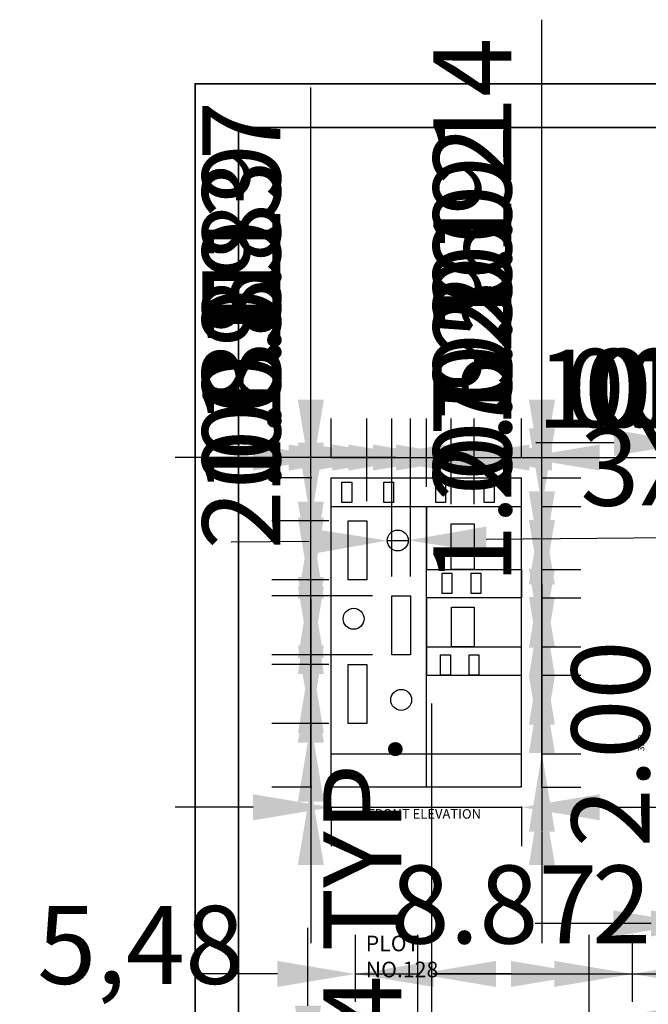
# Model space of a CAD drawing. Units: metres. Extents: x 782 to 1487, y 1262 to 7446.
# Tile 19 of 25: x 782 to 802, y 1313 to 1345. Entities that reach past the tile are written whole.
import ezdxf

# ---------------------------------------------------------------- set-up
doc = ezdxf.new("R2010")
doc.units = ezdxf.units.M
for name, color, linetype, lineweight in [('A-ANNO-DIMS', 2, 'Continuous', 18), ('A-ANNO-TEXT', 3, 'Continuous', 18), ('A-ANNO-TTLB', 7, 'Continuous', 35), ('A-ELEV', 7, 'Continuous', 25)]:
    doc.layers.add(name, color=color, linetype=linetype, lineweight=lineweight)
doc.styles.get("Standard").update_dxf_attribs({"font": 'arial.ttf'})
doc.dimstyles.new('ISO-25', dxfattribs={"dimtxt": 2.5, "dimasz": 2.5, "dimexe": 1.25, "dimexo": 0.625, "dimtad": 1, "dimtxsty": 'Standard', "dimcen": 2.5, "dimadec": 0, "dimazin": 0, "dimtfac": 1, "dimtmove": 0, "dimatfit": 3, "dimfxl": 1, "dimarcsym": 0})

# ---------------------------------------------------------------- blocks, each defined once
blk = doc.blocks.new('*D2')
at = {"layer": 'A-ANNO-DIMS', "color": 0, "lineweight": -2, "transparency": 16777216}
for p, q in [((794.559, 1311.575), (794.559, 1314.2)), ((800.039, 1311.575), (800.039, 1314.2)), ((792.059, 1312.95), (781.81, 1312.95)), ((800.039, 1312.95), (794.559, 1312.95)), ((802.539, 1312.95), (805.039, 1312.95))]:
    blk.add_line(p, q, dxfattribs=at)
at = {"layer": 'A-ANNO-DIMS', "color": 0, "transparency": 16777216}
for points in [[(792.059, 1313.367), (792.059, 1312.534), (794.559, 1312.95)], [(802.539, 1313.367), (802.539, 1312.534), (800.039, 1312.95)]]:
    blk.add_solid(points, dxfattribs=at)
at = {"layer": 'Defpoints', "color": 0, "transparency": 16777216}
for p in [(794.559, 1312.95), (794.559, 1310.95), (800.039, 1310.95)]:
    blk.add_point(p, dxfattribs=at)
at = {"layer": 'A-ANNO-DIMS', "color": 0, "transparency": 16777216, "insert": (785.685, 1315.078), "char_height": 2.5, "width": 6.51678, "attachment_point": 5}
blk.add_mtext('5,48', dxfattribs=at)
blk = doc.blocks.new('*D31')
at = {"layer": 'A-ANNO-DIMS', "color": 0, "lineweight": -2, "transparency": 16777216}
for p, q in [((795.004, 1304.305), (795.004, 1323.137)), ((795.004, 1301.469), (795.004, 1301.805)), ((795.571, 1301.805), (796.254, 1301.805)), ((795.571, 1301.469), (796.254, 1301.469)), ((795.004, 1298.969), (795.004, 1296.469))]:
    blk.add_line(p, q, dxfattribs=at)
at = {"layer": 'A-ANNO-DIMS', "color": 0, "transparency": 16777216}
for points in [[(794.587, 1304.305), (795.421, 1304.305), (795.004, 1301.805)], [(794.587, 1298.969), (795.421, 1298.969), (795.004, 1301.469)]]:
    blk.add_solid(points, dxfattribs=at)
at = {"layer": 'Defpoints', "color": 0, "transparency": 16777216}
for p in [(794.946, 1301.805), (795.004, 1301.805), (794.946, 1301.469)]:
    blk.add_point(p, dxfattribs=at)
at = {"layer": 'A-ANNO-DIMS', "color": 0, "transparency": 16777216, "insert": (793.102, 1314.971), "char_height": 2.5, "attachment_point": 5, "rotation": 90}
blk.add_mtext('0.34 TYP.', dxfattribs=at)
blk = doc.blocks.new('*D32')
at = {"layer": 'A-ANNO-DIMS', "color": 0, "lineweight": -2, "transparency": 16777216}
for p, q in [((791.039, 1313.45), (791.039, 1315.95)), ((793.934, 1310.95), (789.789, 1310.95)), ((791.039, 1310.95), (791.039, 1306.772)), ((793.934, 1306.772), (789.789, 1306.772)), ((791.039, 1304.272), (791.039, 1291.98))]:
    blk.add_line(p, q, dxfattribs=at)
at = {"layer": 'A-ANNO-DIMS', "color": 0, "transparency": 16777216}
for points in [[(790.622, 1313.45), (791.456, 1313.45), (791.039, 1310.95)], [(790.622, 1304.272), (791.456, 1304.272), (791.039, 1306.772)]]:
    blk.add_solid(points, dxfattribs=at)
at = {"layer": 'Defpoints', "color": 0, "transparency": 16777216}
for p in [(794.559, 1310.95), (791.039, 1306.772), (794.559, 1306.772)]:
    blk.add_point(p, dxfattribs=at)
at = {"layer": 'A-ANNO-DIMS', "color": 0, "transparency": 16777216, "insert": (789.138, 1296.876), "char_height": 2.5, "attachment_point": 5, "rotation": 90}
blk.add_mtext('4.178', dxfattribs=at)
blk = doc.blocks.new('*D37')
at = {"layer": 'A-ANNO-DIMS', "color": 0, "lineweight": -2, "transparency": 16777216}
for p, q in [((802.949, 1313.45), (802.949, 1315.95)), ((800.664, 1310.95), (804.199, 1310.95)), ((802.949, 1310.95), (802.949, 1307.03)), ((800.653, 1307.03), (804.199, 1307.03)), ((802.949, 1304.53), (802.949, 1294.314))]:
    blk.add_line(p, q, dxfattribs=at)
at = {"layer": 'A-ANNO-DIMS', "color": 0, "transparency": 16777216}
for points in [[(802.532, 1313.45), (803.366, 1313.45), (802.949, 1310.95)], [(802.532, 1304.53), (803.366, 1304.53), (802.949, 1307.03)]]:
    blk.add_solid(points, dxfattribs=at)
at = {"layer": 'Defpoints', "color": 0, "transparency": 16777216}
for p in [(800.039, 1310.95), (800.028, 1307.03), (802.949, 1307.03)]:
    blk.add_point(p, dxfattribs=at)
at = {"layer": 'A-ANNO-DIMS', "color": 0, "transparency": 16777216, "insert": (801.047, 1298.172), "char_height": 2.5, "attachment_point": 5, "rotation": 90}
blk.add_mtext('3.92', dxfattribs=at)
blk = doc.blocks.new('*D42')
at = {"layer": 'A-ANNO-DIMS', "color": 0, "lineweight": -2, "transparency": 16777216}
for p, q in [((792.559, 1313.575), (792.559, 1315.72)), ((801.429, 1313.575), (801.429, 1315.72)), ((795.059, 1314.47), (798.929, 1314.47))]:
    blk.add_line(p, q, dxfattribs=at)
at = {"layer": 'A-ANNO-DIMS', "color": 0, "transparency": 16777216}
for points in [[(795.059, 1314.887), (795.059, 1314.054), (792.559, 1314.47)], [(798.929, 1314.887), (798.929, 1314.054), (801.429, 1314.47)]]:
    blk.add_solid(points, dxfattribs=at)
at = {"layer": 'Defpoints', "color": 0, "transparency": 16777216}
for p in [(801.429, 1314.47), (792.559, 1312.95), (801.429, 1312.95)]:
    blk.add_point(p, dxfattribs=at)
at = {"layer": 'A-ANNO-DIMS', "color": 0, "transparency": 16777216, "insert": (796.994, 1316.372), "char_height": 2.5, "attachment_point": 5}
blk.add_mtext('8.87', dxfattribs=at)
blk = doc.blocks.new('*D43')
at = {"layer": 'A-ANNO-DIMS', "color": 0, "lineweight": -2, "transparency": 16777216}
for p, q in [((792.559, 1313.575), (792.559, 1315.72)), ((794.559, 1311.575), (794.559, 1315.72)), ((790.059, 1314.47), (787.559, 1314.47)), ((792.559, 1314.47), (794.559, 1314.47)), ((797.059, 1314.47), (807.337, 1314.47))]:
    blk.add_line(p, q, dxfattribs=at)
at = {"layer": 'A-ANNO-DIMS', "color": 0, "transparency": 16777216}
for points in [[(790.059, 1314.887), (790.059, 1314.054), (792.559, 1314.47)], [(797.059, 1314.887), (797.059, 1314.054), (794.559, 1314.47)]]:
    blk.add_solid(points, dxfattribs=at)
at = {"layer": 'Defpoints', "color": 0, "transparency": 16777216}
for p in [(794.559, 1314.47), (792.559, 1312.95), (794.559, 1310.95)]:
    blk.add_point(p, dxfattribs=at)
at = {"layer": 'A-ANNO-DIMS', "color": 0, "transparency": 16777216, "insert": (803.448, 1316.372), "char_height": 2.5, "attachment_point": 5}
blk.add_mtext('2.00', dxfattribs=at)
blk = doc.blocks.new('*D44')
at = {"layer": 'A-ANNO-DIMS', "color": 0, "lineweight": -2, "transparency": 16777216}
for p, q in [((800.039, 1311.575), (800.039, 1315.72)), ((801.429, 1313.575), (801.429, 1315.72)), ((797.539, 1314.47), (795.039, 1314.47)), ((800.039, 1314.47), (801.429, 1314.47)), ((803.929, 1314.47), (813.943, 1314.47))]:
    blk.add_line(p, q, dxfattribs=at)
at = {"layer": 'A-ANNO-DIMS', "color": 0, "transparency": 16777216}
for points in [[(797.539, 1314.887), (797.539, 1314.054), (800.039, 1314.47)], [(803.929, 1314.887), (803.929, 1314.054), (801.429, 1314.47)]]:
    blk.add_solid(points, dxfattribs=at)
at = {"layer": 'Defpoints', "color": 0, "transparency": 16777216}
for p in [(801.429, 1314.47), (801.429, 1312.95), (800.039, 1310.95)]:
    blk.add_point(p, dxfattribs=at)
at = {"layer": 'A-ANNO-DIMS', "color": 0, "transparency": 16777216, "insert": (810.186, 1316.373), "char_height": 2.5, "attachment_point": 5}
blk.add_mtext('1.39', dxfattribs=at)
blk = doc.blocks.new('*D47')
at = {"layer": 'A-ANNO-DIMS', "color": 0, "lineweight": -2, "transparency": 16777216}
for p, q in [((802.949, 1315.45), (802.949, 1325.728)), ((802.054, 1312.95), (804.199, 1312.95)), ((802.949, 1310.95), (802.949, 1312.95)), ((800.664, 1310.95), (804.199, 1310.95)), ((802.949, 1308.45), (802.949, 1305.95))]:
    blk.add_line(p, q, dxfattribs=at)
at = {"layer": 'A-ANNO-DIMS', "color": 0, "transparency": 16777216}
for points in [[(802.532, 1315.45), (803.366, 1315.45), (802.949, 1312.95)], [(802.532, 1308.45), (803.366, 1308.45), (802.949, 1310.95)]]:
    blk.add_solid(points, dxfattribs=at)
at = {"layer": 'Defpoints', "color": 0, "transparency": 16777216}
for p in [(801.429, 1312.95), (802.949, 1312.95), (800.039, 1310.95)]:
    blk.add_point(p, dxfattribs=at)
at = {"layer": 'A-ANNO-DIMS', "color": 0, "transparency": 16777216, "insert": (801.048, 1321.839), "char_height": 2.5, "attachment_point": 5, "rotation": 90}
blk.add_mtext('2.00', dxfattribs=at)
blk = doc.blocks.new('*D115')
at = {"layer": 'A-ANNO-DIMS', "color": 0, "lineweight": -2, "transparency": 16777216}
for p, q in [((789.282, 1319.809), (786.782, 1319.809)), ((791.782, 1319.834), (791.782, 1318.559)), ((791.782, 1319.809), (797.878, 1319.809)), ((797.878, 1319.834), (797.878, 1318.559)), ((800.378, 1319.809), (812.576, 1319.809))]:
    blk.add_line(p, q, dxfattribs=at)
at = {"layer": 'A-ANNO-DIMS', "color": 0, "transparency": 16777216}
for points in [[(789.282, 1320.226), (789.282, 1319.392), (791.782, 1319.809)], [(800.378, 1320.226), (800.378, 1319.392), (797.878, 1319.809)]]:
    blk.add_solid(points, dxfattribs=at)
at = {"layer": 'Defpoints', "color": 0, "transparency": 16777216}
for p in [(791.782, 1320.459), (797.878, 1320.459), (797.878, 1319.809)]:
    blk.add_point(p, dxfattribs=at)
at = {"layer": 'A-ANNO-DIMS', "color": 0, "transparency": 16777216, "insert": (807.727, 1321.711), "char_height": 2.5, "attachment_point": 5}
blk.add_mtext('6.096', dxfattribs=at)
blk = doc.blocks.new('*D116')
at = {"layer": 'A-ANNO-DIMS', "color": 0, "lineweight": -2, "transparency": 16777216}
for p, q in [((791.782, 1330.988), (791.782, 1332.263)), ((792.923, 1329.614), (792.923, 1332.263)), ((789.282, 1331.013), (786.782, 1331.013)), ((791.782, 1331.013), (792.923, 1331.013)), ((795.423, 1331.013), (805.421, 1331.013))]:
    blk.add_line(p, q, dxfattribs=at)
at = {"layer": 'A-ANNO-DIMS', "color": 0, "transparency": 16777216}
for points in [[(789.282, 1331.43), (789.282, 1330.597), (791.782, 1331.013)], [(795.423, 1331.43), (795.423, 1330.597), (792.923, 1331.013)]]:
    blk.add_solid(points, dxfattribs=at)
at = {"layer": 'Defpoints', "color": 0, "transparency": 16777216}
for p in [(792.923, 1331.013), (791.782, 1330.363), (792.923, 1328.989)]:
    blk.add_point(p, dxfattribs=at)
at = {"layer": 'A-ANNO-DIMS', "color": 0, "transparency": 16777216, "insert": (801.672, 1332.894), "char_height": 2.5, "attachment_point": 5}
blk.add_mtext('1.14', dxfattribs=at)
blk = doc.blocks.new('*D117')
at = {"layer": 'A-ANNO-DIMS', "color": 0, "lineweight": -2, "transparency": 16777216}
for p, q in [((792.923, 1329.614), (792.923, 1332.263)), ((793.726, 1327.207), (793.726, 1332.263)), ((790.423, 1331.013), (787.923, 1331.013)), ((792.923, 1331.013), (793.726, 1331.013)), ((796.226, 1331.013), (806.461, 1331.013))]:
    blk.add_line(p, q, dxfattribs=at)
at = {"layer": 'A-ANNO-DIMS', "color": 0, "transparency": 16777216}
for points in [[(790.423, 1331.43), (790.423, 1330.597), (792.923, 1331.013)], [(796.226, 1331.43), (796.226, 1330.597), (793.726, 1331.013)]]:
    blk.add_solid(points, dxfattribs=at)
at = {"layer": 'Defpoints', "color": 0, "transparency": 16777216}
for p in [(793.726, 1331.013), (792.923, 1328.989), (793.726, 1326.582)]:
    blk.add_point(p, dxfattribs=at)
at = {"layer": 'A-ANNO-DIMS', "color": 0, "transparency": 16777216, "insert": (802.594, 1332.915), "char_height": 2.5, "attachment_point": 5}
blk.add_mtext('0.80', dxfattribs=at)
blk = doc.blocks.new('*D118')
at = {"layer": 'A-ANNO-DIMS', "color": 0, "lineweight": -2, "transparency": 16777216}
for p, q in [((793.726, 1327.207), (793.726, 1332.263)), ((794.32, 1327.207), (794.32, 1332.263)), ((791.226, 1331.013), (788.726, 1331.013)), ((793.726, 1331.013), (794.32, 1331.013)), ((796.82, 1331.013), (807.069, 1331.013))]:
    blk.add_line(p, q, dxfattribs=at)
at = {"layer": 'A-ANNO-DIMS', "color": 0, "transparency": 16777216}
for points in [[(791.226, 1331.43), (791.226, 1330.597), (793.726, 1331.013)], [(796.82, 1331.43), (796.82, 1330.597), (794.32, 1331.013)]]:
    blk.add_solid(points, dxfattribs=at)
at = {"layer": 'Defpoints', "color": 0, "transparency": 16777216}
for p in [(794.32, 1331.013), (793.726, 1326.582), (794.32, 1326.582)]:
    blk.add_point(p, dxfattribs=at)
at = {"layer": 'A-ANNO-DIMS', "color": 0, "transparency": 16777216, "insert": (803.194, 1332.915), "char_height": 2.5, "attachment_point": 5}
blk.add_mtext('0.59', dxfattribs=at)
blk = doc.blocks.new('*D119')
at = {"layer": 'A-ANNO-DIMS', "color": 0, "lineweight": -2, "transparency": 16777216}
for p, q in [((794.32, 1327.207), (794.32, 1332.263)), ((794.83, 1330.074), (794.83, 1332.263)), ((791.82, 1331.013), (789.32, 1331.013)), ((794.32, 1331.013), (794.83, 1331.013)), ((797.33, 1331.013), (807.091, 1331.013))]:
    blk.add_line(p, q, dxfattribs=at)
at = {"layer": 'A-ANNO-DIMS', "color": 0, "transparency": 16777216}
for points in [[(791.82, 1331.43), (791.82, 1330.597), (794.32, 1331.013)], [(797.33, 1331.43), (797.33, 1330.597), (794.83, 1331.013)]]:
    blk.add_solid(points, dxfattribs=at)
at = {"layer": 'Defpoints', "color": 0, "transparency": 16777216}
for p in [(794.83, 1331.013), (794.83, 1329.449), (794.32, 1326.582)]:
    blk.add_point(p, dxfattribs=at)
at = {"layer": 'A-ANNO-DIMS', "color": 0, "transparency": 16777216, "insert": (803.46, 1332.915), "char_height": 2.5, "attachment_point": 5}
blk.add_mtext('0.51', dxfattribs=at)
blk = doc.blocks.new('*D120')
at = {"layer": 'A-ANNO-DIMS', "color": 0, "lineweight": -2, "transparency": 16777216}
for p, q in [((794.83, 1330.074), (794.83, 1332.263)), ((795.62, 1329.519), (795.62, 1332.263)), ((792.33, 1331.013), (789.83, 1331.013)), ((794.83, 1331.013), (795.62, 1331.013)), ((798.12, 1331.013), (808.369, 1331.013))]:
    blk.add_line(p, q, dxfattribs=at)
at = {"layer": 'A-ANNO-DIMS', "color": 0, "transparency": 16777216}
for points in [[(792.33, 1331.43), (792.33, 1330.597), (794.83, 1331.013)], [(798.12, 1331.43), (798.12, 1330.597), (795.62, 1331.013)]]:
    blk.add_solid(points, dxfattribs=at)
at = {"layer": 'Defpoints', "color": 0, "transparency": 16777216}
for p in [(795.62, 1331.013), (794.83, 1329.449), (795.62, 1328.894)]:
    blk.add_point(p, dxfattribs=at)
at = {"layer": 'A-ANNO-DIMS', "color": 0, "transparency": 16777216, "insert": (804.495, 1332.915), "char_height": 2.5, "attachment_point": 5}
blk.add_mtext('0.79', dxfattribs=at)
blk = doc.blocks.new('*D121')
at = {"layer": 'A-ANNO-DIMS', "color": 0, "lineweight": -2, "transparency": 16777216}
for p, q in [((795.62, 1329.519), (795.62, 1332.263)), ((796.354, 1329.519), (796.354, 1332.263)), ((793.12, 1331.013), (790.62, 1331.013)), ((795.62, 1331.013), (796.354, 1331.013)), ((798.854, 1331.013), (809.098, 1331.013))]:
    blk.add_line(p, q, dxfattribs=at)
at = {"layer": 'A-ANNO-DIMS', "color": 0, "transparency": 16777216}
for points in [[(793.12, 1331.43), (793.12, 1330.597), (795.62, 1331.013)], [(798.854, 1331.43), (798.854, 1330.597), (796.354, 1331.013)]]:
    blk.add_solid(points, dxfattribs=at)
at = {"layer": 'Defpoints', "color": 0, "transparency": 16777216}
for p in [(796.354, 1331.013), (795.62, 1328.894), (796.354, 1328.894)]:
    blk.add_point(p, dxfattribs=at)
at = {"layer": 'A-ANNO-DIMS', "color": 0, "transparency": 16777216, "insert": (805.226, 1332.916), "char_height": 2.5, "attachment_point": 5}
blk.add_mtext('0.73', dxfattribs=at)
blk = doc.blocks.new('*D122')
at = {"layer": 'A-ANNO-DIMS', "color": 0, "lineweight": -2, "transparency": 16777216}
for p, q in [((796.354, 1329.519), (796.354, 1332.263)), ((797.878, 1330.988), (797.878, 1332.263)), ((793.854, 1331.013), (791.354, 1331.013)), ((796.354, 1331.013), (797.878, 1331.013)), ((800.378, 1331.013), (812.318, 1331.013))]:
    blk.add_line(p, q, dxfattribs=at)
at = {"layer": 'A-ANNO-DIMS', "color": 0, "transparency": 16777216}
for points in [[(793.854, 1331.43), (793.854, 1330.597), (796.354, 1331.013)], [(800.378, 1331.43), (800.378, 1330.597), (797.878, 1331.013)]]:
    blk.add_solid(points, dxfattribs=at)
at = {"layer": 'Defpoints', "color": 0, "transparency": 16777216}
for p in [(797.878, 1331.013), (797.878, 1330.363), (796.354, 1328.894)]:
    blk.add_point(p, dxfattribs=at)
at = {"layer": 'A-ANNO-DIMS', "color": 0, "transparency": 16777216, "insert": (807.598, 1332.915), "char_height": 2.5, "attachment_point": 5}
blk.add_mtext('1.524', dxfattribs=at)
blk = doc.blocks.new('*D123')
at = {"layer": 'A-ANNO-DIMS', "color": 0, "lineweight": -2, "transparency": 16777216}
for p, q in [((791.132, 1324.989), (791.132, 1335.276)), ((791.704, 1322.489), (789.882, 1322.489)), ((791.132, 1320.459), (791.132, 1322.489)), ((791.157, 1320.459), (789.882, 1320.459)), ((791.132, 1317.959), (791.132, 1315.459))]:
    blk.add_line(p, q, dxfattribs=at)
at = {"layer": 'A-ANNO-DIMS', "color": 0, "transparency": 16777216}
for points in [[(790.715, 1324.989), (791.548, 1324.989), (791.132, 1322.489)], [(790.715, 1317.959), (791.548, 1317.959), (791.132, 1320.459)]]:
    blk.add_solid(points, dxfattribs=at)
at = {"layer": 'Defpoints', "color": 0, "transparency": 16777216}
for p in [(791.132, 1322.489), (792.329, 1322.489), (791.782, 1320.459)]:
    blk.add_point(p, dxfattribs=at)
at = {"layer": 'A-ANNO-DIMS', "color": 0, "transparency": 16777216, "insert": (789.23, 1331.382), "char_height": 2.5, "attachment_point": 5, "rotation": 90}
blk.add_mtext('2.03', dxfattribs=at)
blk = doc.blocks.new('*D124')
at = {"layer": 'A-ANNO-DIMS', "color": 0, "lineweight": -2, "transparency": 16777216}
for p, q in [((791.132, 1326.882), (791.132, 1336.896)), ((791.704, 1324.382), (789.882, 1324.382)), ((791.132, 1322.489), (791.132, 1324.382)), ((791.704, 1322.489), (789.882, 1322.489)), ((791.132, 1319.989), (791.132, 1317.489))]:
    blk.add_line(p, q, dxfattribs=at)
at = {"layer": 'A-ANNO-DIMS', "color": 0, "transparency": 16777216}
for points in [[(790.715, 1326.882), (791.548, 1326.882), (791.132, 1324.382)], [(790.715, 1319.989), (791.548, 1319.989), (791.132, 1322.489)]]:
    blk.add_solid(points, dxfattribs=at)
at = {"layer": 'Defpoints', "color": 0, "transparency": 16777216}
for p in [(791.132, 1324.382), (792.329, 1324.382), (792.329, 1322.489)]:
    blk.add_point(p, dxfattribs=at)
at = {"layer": 'A-ANNO-DIMS', "color": 0, "transparency": 16777216, "insert": (789.23, 1333.139), "char_height": 2.5, "attachment_point": 5, "rotation": 90}
blk.add_mtext('1.89', dxfattribs=at)
blk = doc.blocks.new('*D125')
at = {"layer": 'A-ANNO-DIMS', "color": 0, "lineweight": -2, "transparency": 16777216}
for p, q in [((791.132, 1327.189), (791.132, 1336.95)), ((793.101, 1324.689), (789.882, 1324.689)), ((791.132, 1324.382), (791.132, 1324.689)), ((791.704, 1324.382), (789.882, 1324.382)), ((791.132, 1321.882), (791.132, 1319.382))]:
    blk.add_line(p, q, dxfattribs=at)
at = {"layer": 'A-ANNO-DIMS', "color": 0, "transparency": 16777216}
for points in [[(790.715, 1327.189), (791.548, 1327.189), (791.132, 1324.689)], [(790.715, 1321.882), (791.548, 1321.882), (791.132, 1324.382)]]:
    blk.add_solid(points, dxfattribs=at)
at = {"layer": 'Defpoints', "color": 0, "transparency": 16777216}
for p in [(791.132, 1324.689), (793.726, 1324.689), (792.329, 1324.382)]:
    blk.add_point(p, dxfattribs=at)
at = {"layer": 'A-ANNO-DIMS', "color": 0, "transparency": 16777216, "insert": (789.23, 1333.32), "char_height": 2.5, "attachment_point": 5, "rotation": 90}
blk.add_mtext('0.31', dxfattribs=at)
blk = doc.blocks.new('*D126')
at = {"layer": 'A-ANNO-DIMS', "color": 0, "lineweight": -2, "transparency": 16777216}
for p, q in [((791.132, 1329.082), (791.132, 1339.096)), ((793.101, 1326.582), (789.882, 1326.582)), ((791.132, 1324.689), (791.132, 1326.582)), ((793.101, 1324.689), (789.882, 1324.689)), ((791.132, 1322.189), (791.132, 1319.689))]:
    blk.add_line(p, q, dxfattribs=at)
at = {"layer": 'A-ANNO-DIMS', "color": 0, "transparency": 16777216}
for points in [[(790.715, 1329.082), (791.548, 1329.082), (791.132, 1326.582)], [(790.715, 1322.189), (791.548, 1322.189), (791.132, 1324.689)]]:
    blk.add_solid(points, dxfattribs=at)
at = {"layer": 'Defpoints', "color": 0, "transparency": 16777216}
for p in [(791.132, 1326.582), (793.726, 1326.582), (793.726, 1324.689)]:
    blk.add_point(p, dxfattribs=at)
at = {"layer": 'A-ANNO-DIMS', "color": 0, "transparency": 16777216, "insert": (789.23, 1335.339), "char_height": 2.5, "attachment_point": 5, "rotation": 90}
blk.add_mtext('1.89', dxfattribs=at)
blk = doc.blocks.new('*D127')
at = {"layer": 'A-ANNO-DIMS', "color": 0, "lineweight": -2, "transparency": 16777216}
for p, q in [((791.132, 1329.596), (791.132, 1339.357)), ((791.704, 1327.096), (789.882, 1327.096)), ((791.132, 1326.582), (791.132, 1327.096)), ((793.101, 1326.582), (789.882, 1326.582)), ((791.132, 1324.082), (791.132, 1321.582))]:
    blk.add_line(p, q, dxfattribs=at)
at = {"layer": 'A-ANNO-DIMS', "color": 0, "transparency": 16777216}
for points in [[(790.715, 1329.596), (791.548, 1329.596), (791.132, 1327.096)], [(790.715, 1324.082), (791.548, 1324.082), (791.132, 1326.582)]]:
    blk.add_solid(points, dxfattribs=at)
at = {"layer": 'Defpoints', "color": 0, "transparency": 16777216}
for p in [(791.132, 1327.096), (792.329, 1327.096), (793.726, 1326.582)]:
    blk.add_point(p, dxfattribs=at)
at = {"layer": 'A-ANNO-DIMS', "color": 0, "transparency": 16777216, "insert": (789.23, 1335.726), "char_height": 2.5, "attachment_point": 5, "rotation": 90}
blk.add_mtext('0.51', dxfattribs=at)
blk = doc.blocks.new('*D128')
at = {"layer": 'A-ANNO-DIMS', "color": 0, "lineweight": -2, "transparency": 16777216}
for p, q in [((791.132, 1331.489), (791.132, 1341.503)), ((791.704, 1328.989), (789.882, 1328.989)), ((791.132, 1327.096), (791.132, 1328.989)), ((791.704, 1327.096), (789.882, 1327.096)), ((791.132, 1324.596), (791.132, 1322.096))]:
    blk.add_line(p, q, dxfattribs=at)
at = {"layer": 'A-ANNO-DIMS', "color": 0, "transparency": 16777216}
for points in [[(790.715, 1331.489), (791.548, 1331.489), (791.132, 1328.989)], [(790.715, 1324.596), (791.548, 1324.596), (791.132, 1327.096)]]:
    blk.add_solid(points, dxfattribs=at)
at = {"layer": 'Defpoints', "color": 0, "transparency": 16777216}
for p in [(791.132, 1328.989), (792.329, 1328.989), (792.329, 1327.096)]:
    blk.add_point(p, dxfattribs=at)
at = {"layer": 'A-ANNO-DIMS', "color": 0, "transparency": 16777216, "insert": (789.23, 1337.746), "char_height": 2.5, "attachment_point": 5, "rotation": 90}
blk.add_mtext('1.89', dxfattribs=at)
blk = doc.blocks.new('*D129')
at = {"layer": 'A-ANNO-DIMS', "color": 0, "lineweight": -2, "transparency": 16777216}
for p, q in [((791.132, 1332.863), (791.132, 1342.872)), ((791.157, 1330.363), (789.882, 1330.363)), ((791.132, 1328.989), (791.132, 1330.363)), ((791.704, 1328.989), (789.882, 1328.989)), ((791.132, 1326.489), (791.132, 1323.989))]:
    blk.add_line(p, q, dxfattribs=at)
at = {"layer": 'A-ANNO-DIMS', "color": 0, "transparency": 16777216}
for points in [[(790.715, 1332.863), (791.548, 1332.863), (791.132, 1330.363)], [(790.715, 1326.489), (791.548, 1326.489), (791.132, 1328.989)]]:
    blk.add_solid(points, dxfattribs=at)
at = {"layer": 'Defpoints', "color": 0, "transparency": 16777216}
for p in [(791.132, 1330.363), (791.782, 1330.363), (792.329, 1328.989)]:
    blk.add_point(p, dxfattribs=at)
at = {"layer": 'A-ANNO-DIMS', "color": 0, "transparency": 16777216, "insert": (789.23, 1339.118), "char_height": 2.5, "attachment_point": 5, "rotation": 90}
blk.add_mtext('1.37', dxfattribs=at)
blk = doc.blocks.new('*D130')
at = {"layer": 'A-ANNO-DIMS', "color": 0, "lineweight": -2, "transparency": 16777216}
for p, q in [((798.528, 1324.025), (798.528, 1334.034)), ((798.503, 1321.525), (799.778, 1321.525)), ((798.528, 1320.459), (798.528, 1321.525)), ((798.503, 1320.459), (799.778, 1320.459)), ((798.528, 1317.959), (798.528, 1315.459))]:
    blk.add_line(p, q, dxfattribs=at)
at = {"layer": 'A-ANNO-DIMS', "color": 0, "transparency": 16777216}
for points in [[(798.111, 1324.025), (798.944, 1324.025), (798.528, 1321.525)], [(798.111, 1317.959), (798.944, 1317.959), (798.528, 1320.459)]]:
    blk.add_solid(points, dxfattribs=at)
at = {"layer": 'Defpoints', "color": 0, "transparency": 16777216}
for p in [(797.878, 1321.525), (798.528, 1321.525), (797.878, 1320.459)]:
    blk.add_point(p, dxfattribs=at)
at = {"layer": 'A-ANNO-DIMS', "color": 0, "transparency": 16777216, "insert": (796.626, 1330.28), "char_height": 2.5, "attachment_point": 5, "rotation": 90}
blk.add_mtext('1.07', dxfattribs=at)
blk = doc.blocks.new('*D131')
at = {"layer": 'A-ANNO-DIMS', "color": 0, "lineweight": -2, "transparency": 16777216}
for p, q in [((798.528, 1326.546), (798.528, 1336.807)), ((798.503, 1324.046), (799.778, 1324.046)), ((798.528, 1321.525), (798.528, 1324.046)), ((798.503, 1321.525), (799.778, 1321.525)), ((798.528, 1319.025), (798.528, 1316.525))]:
    blk.add_line(p, q, dxfattribs=at)
at = {"layer": 'A-ANNO-DIMS', "color": 0, "transparency": 16777216}
for points in [[(798.111, 1326.546), (798.944, 1326.546), (798.528, 1324.046)], [(798.111, 1319.025), (798.944, 1319.025), (798.528, 1321.525)]]:
    blk.add_solid(points, dxfattribs=at)
at = {"layer": 'Defpoints', "color": 0, "transparency": 16777216}
for p in [(797.878, 1324.046), (798.528, 1324.046), (797.878, 1321.525)]:
    blk.add_point(p, dxfattribs=at)
at = {"layer": 'A-ANNO-DIMS', "color": 0, "transparency": 16777216, "insert": (796.626, 1332.927), "char_height": 2.5, "attachment_point": 5, "rotation": 90}
blk.add_mtext('2.52', dxfattribs=at)
blk = doc.blocks.new('*D132')
at = {"layer": 'A-ANNO-DIMS', "color": 0, "lineweight": -2, "transparency": 16777216}
for p, q in [((798.528, 1327.454), (798.528, 1337.216)), ((798.503, 1324.954), (799.778, 1324.954)), ((798.528, 1324.046), (798.528, 1324.954)), ((798.503, 1324.046), (799.778, 1324.046)), ((798.528, 1321.546), (798.528, 1319.046))]:
    blk.add_line(p, q, dxfattribs=at)
at = {"layer": 'A-ANNO-DIMS', "color": 0, "transparency": 16777216}
for points in [[(798.111, 1327.454), (798.944, 1327.454), (798.528, 1324.954)], [(798.111, 1321.546), (798.944, 1321.546), (798.528, 1324.046)]]:
    blk.add_solid(points, dxfattribs=at)
at = {"layer": 'Defpoints', "color": 0, "transparency": 16777216}
for p in [(797.878, 1324.954), (798.528, 1324.954), (797.878, 1324.046)]:
    blk.add_point(p, dxfattribs=at)
at = {"layer": 'A-ANNO-DIMS', "color": 0, "transparency": 16777216, "insert": (796.626, 1333.585), "char_height": 2.5, "attachment_point": 5, "rotation": 90}
blk.add_mtext('0.91', dxfattribs=at)
blk = doc.blocks.new('*D133')
at = {"layer": 'A-ANNO-DIMS', "color": 0, "lineweight": -2, "transparency": 16777216}
for p, q in [((798.528, 1329.015), (798.528, 1339.021)), ((798.503, 1326.515), (799.778, 1326.515)), ((798.528, 1324.954), (798.528, 1326.515)), ((798.503, 1324.954), (799.778, 1324.954)), ((798.528, 1322.454), (798.528, 1319.954))]:
    blk.add_line(p, q, dxfattribs=at)
at = {"layer": 'A-ANNO-DIMS', "color": 0, "transparency": 16777216}
for points in [[(798.111, 1329.015), (798.944, 1329.015), (798.528, 1326.515)], [(798.111, 1322.454), (798.944, 1322.454), (798.528, 1324.954)]]:
    blk.add_solid(points, dxfattribs=at)
at = {"layer": 'Defpoints', "color": 0, "transparency": 16777216}
for p in [(797.878, 1326.515), (798.528, 1326.515), (797.878, 1324.954)]:
    blk.add_point(p, dxfattribs=at)
at = {"layer": 'A-ANNO-DIMS', "color": 0, "transparency": 16777216, "insert": (796.626, 1335.268), "char_height": 2.5, "attachment_point": 5, "rotation": 90}
blk.add_mtext('1.56', dxfattribs=at)
blk = doc.blocks.new('*D134')
at = {"layer": 'A-ANNO-DIMS', "color": 0, "lineweight": -2, "transparency": 16777216}
for p, q in [((798.528, 1329.926), (798.528, 1339.688)), ((798.503, 1327.426), (799.778, 1327.426)), ((798.528, 1326.515), (798.528, 1327.426)), ((798.503, 1326.515), (799.778, 1326.515)), ((798.528, 1324.015), (798.528, 1321.515))]:
    blk.add_line(p, q, dxfattribs=at)
at = {"layer": 'A-ANNO-DIMS', "color": 0, "transparency": 16777216}
for points in [[(798.111, 1329.926), (798.944, 1329.926), (798.528, 1327.426)], [(798.111, 1324.015), (798.944, 1324.015), (798.528, 1326.515)]]:
    blk.add_solid(points, dxfattribs=at)
at = {"layer": 'Defpoints', "color": 0, "transparency": 16777216}
for p in [(797.878, 1327.426), (798.528, 1327.426), (797.878, 1326.515)]:
    blk.add_point(p, dxfattribs=at)
at = {"layer": 'A-ANNO-DIMS', "color": 0, "transparency": 16777216, "insert": (796.626, 1336.057), "char_height": 2.5, "attachment_point": 5, "rotation": 90}
blk.add_mtext('0.91', dxfattribs=at)
blk = doc.blocks.new('*D135')
at = {"layer": 'A-ANNO-DIMS', "color": 0, "lineweight": -2, "transparency": 16777216}
for p, q in [((798.528, 1331.949), (798.528, 1342.21)), ((798.503, 1329.449), (799.778, 1329.449)), ((798.528, 1327.426), (798.528, 1329.449)), ((798.503, 1327.426), (799.778, 1327.426)), ((798.528, 1324.926), (798.528, 1322.426))]:
    blk.add_line(p, q, dxfattribs=at)
at = {"layer": 'A-ANNO-DIMS', "color": 0, "transparency": 16777216}
for points in [[(798.111, 1331.949), (798.944, 1331.949), (798.528, 1329.449)], [(798.111, 1324.926), (798.944, 1324.926), (798.528, 1327.426)]]:
    blk.add_solid(points, dxfattribs=at)
at = {"layer": 'Defpoints', "color": 0, "transparency": 16777216}
for p in [(797.878, 1329.449), (798.528, 1329.449), (797.878, 1327.426)]:
    blk.add_point(p, dxfattribs=at)
at = {"layer": 'A-ANNO-DIMS', "color": 0, "transparency": 16777216, "insert": (796.626, 1338.33), "char_height": 2.5, "attachment_point": 5, "rotation": 90}
blk.add_mtext('2.02', dxfattribs=at)
blk = doc.blocks.new('*D136')
at = {"layer": 'A-ANNO-DIMS', "color": 0, "lineweight": -2, "transparency": 16777216}
for p, q in [((798.528, 1332.863), (798.528, 1345.039)), ((798.503, 1330.363), (799.778, 1330.363)), ((798.528, 1329.449), (798.528, 1330.363)), ((798.503, 1329.449), (799.778, 1329.449)), ((798.528, 1326.949), (798.528, 1324.449))]:
    blk.add_line(p, q, dxfattribs=at)
at = {"layer": 'A-ANNO-DIMS', "color": 0, "transparency": 16777216}
for points in [[(798.111, 1332.863), (798.944, 1332.863), (798.528, 1330.363)], [(798.111, 1326.949), (798.944, 1326.949), (798.528, 1329.449)]]:
    blk.add_solid(points, dxfattribs=at)
at = {"layer": 'Defpoints', "color": 0, "transparency": 16777216}
for p in [(797.878, 1330.363), (798.528, 1330.363), (797.878, 1329.449)]:
    blk.add_point(p, dxfattribs=at)
at = {"layer": 'A-ANNO-DIMS', "color": 0, "transparency": 16777216, "insert": (796.626, 1340.201), "char_height": 2.5, "attachment_point": 5, "rotation": 90}
blk.add_mtext('0.914', dxfattribs=at)
blk = doc.blocks.new('*D138')
at = {"layer": 'A-ANNO-DIMS', "color": 0, "lineweight": -2, "transparency": 16777216}
for p, q in [((803.332, 1330.988), (803.332, 1332.733)), ((803.562, 1330.988), (803.562, 1332.733)), ((800.832, 1331.483), (798.332, 1331.483)), ((803.332, 1331.483), (803.562, 1331.483)), ((806.062, 1331.483), (816.306, 1331.483))]:
    blk.add_line(p, q, dxfattribs=at)
at = {"layer": 'A-ANNO-DIMS', "color": 0, "transparency": 16777216}
for points in [[(800.832, 1331.899), (800.832, 1331.066), (803.332, 1331.483)], [(806.062, 1331.899), (806.062, 1331.066), (803.562, 1331.483)]]:
    blk.add_solid(points, dxfattribs=at)
at = {"layer": 'Defpoints', "color": 0, "transparency": 16777216}
for p in [(803.562, 1331.483), (803.332, 1330.363), (803.562, 1330.363)]:
    blk.add_point(p, dxfattribs=at)
at = {"layer": 'A-ANNO-DIMS', "color": 0, "transparency": 16777216, "insert": (812.434, 1333.385), "char_height": 2.5, "attachment_point": 5}
blk.add_mtext('0.23', dxfattribs=at)
blk = doc.blocks.new('*D140')
at = {"layer": 'A-ANNO-DIMS', "color": 0, "lineweight": -2, "transparency": 16777216}
for p, q in [((803.316, 1317.905), (803.316, 1314.838)), ((804.52, 1317.905), (804.52, 1314.838)), ((800.816, 1316.088), (798.316, 1316.088)), ((803.316, 1316.088), (804.52, 1316.088)), ((807.02, 1316.088), (817.02, 1316.088))]:
    blk.add_line(p, q, dxfattribs=at)
at = {"layer": 'A-ANNO-DIMS', "color": 0, "transparency": 16777216}
for points in [[(800.816, 1316.505), (800.816, 1315.671), (803.316, 1316.088)], [(807.02, 1316.505), (807.02, 1315.671), (804.52, 1316.088)]]:
    blk.add_solid(points, dxfattribs=at)
at = {"layer": 'Defpoints', "color": 0, "transparency": 16777216}
for p in [(803.316, 1318.53), (804.52, 1318.53), (804.52, 1316.088)]:
    blk.add_point(p, dxfattribs=at)
at = {"layer": 'A-ANNO-DIMS', "color": 0, "transparency": 16777216, "insert": (813.27, 1317.989), "char_height": 2.5, "attachment_point": 5}
blk.add_mtext('1.20', dxfattribs=at)
blk = doc.blocks.new('*D141')
at = {"layer": 'A-ANNO-DIMS', "color": 0, "lineweight": -2, "transparency": 16777216}
for p, q in [((804.52, 1317.905), (804.52, 1314.838)), ((807.205, 1317.905), (807.205, 1314.838)), ((802.02, 1316.088), (799.52, 1316.088)), ((804.52, 1316.088), (807.205, 1316.088)), ((809.705, 1316.088), (819.997, 1316.088))]:
    blk.add_line(p, q, dxfattribs=at)
at = {"layer": 'A-ANNO-DIMS', "color": 0, "transparency": 16777216}
for points in [[(802.02, 1316.505), (802.02, 1315.671), (804.52, 1316.088)], [(809.705, 1316.505), (809.705, 1315.671), (807.205, 1316.088)]]:
    blk.add_solid(points, dxfattribs=at)
at = {"layer": 'Defpoints', "color": 0, "transparency": 16777216}
for p in [(804.52, 1318.53), (807.205, 1318.53), (807.205, 1316.088)]:
    blk.add_point(p, dxfattribs=at)
at = {"layer": 'A-ANNO-DIMS', "color": 0, "transparency": 16777216, "insert": (816.101, 1317.989), "char_height": 2.5, "attachment_point": 5}
blk.add_mtext('2.68', dxfattribs=at)
blk = doc.blocks.new('*D170')
at = {"layer": 'A-ANNO-DIMS', "color": 0, "lineweight": -2, "transparency": 16777216}
for p, q in [((814.947, 1328.566), (796.747, 1328.385)), ((791.077, 1328.328), (788.578, 1328.304)), ((793.577, 1328.353), (794.248, 1328.36))]:
    blk.add_line(p, q, dxfattribs=at)
at = {"layer": 'A-ANNO-DIMS', "color": 0, "transparency": 16777216}
for points in [[(791.073, 1328.745), (791.082, 1327.912), (793.577, 1328.353)], [(796.743, 1328.802), (796.752, 1327.968), (794.248, 1328.36)]]:
    blk.add_solid(points, dxfattribs=at)
at = {"layer": 'Defpoints', "color": 0, "transparency": 16777216}
for p in [(793.577, 1328.353), (794.248, 1328.36)]:
    blk.add_point(p, dxfattribs=at)
at = {"layer": 'A-ANNO-DIMS', "color": 0, "transparency": 16777216, "insert": (807.078, 1330.459), "char_height": 2.5, "attachment_point": 5, "rotation": 0.5708}
blk.add_mtext('3X ∅0.67', dxfattribs=at)

msp = doc.modelspace()

# ---------------------------------------------------------------- linework, layer by layer
at = {"layer": 'A-ANNO-TTLB'}
for points in [[(787.4248, 1342.9861), (880.8003, 1342.9861), (880.8003, 1263.8004), (787.4248, 1263.8004)], [(883.6865, 1262.3458), (787.4248, 1262.3458), (787.4248, 1342.9861), (883.6865, 1342.9861)], [(788.8147, 1341.5907), (880.8003, 1341.5907), (880.8003, 1263.8004), (788.8147, 1263.8004)]]:
    msp.add_lwpolyline(points, close=True, dxfattribs=at)
at = {"layer": 'A-ELEV'}
for p, q in [((791.7818, 1330.3635), (797.8778, 1330.3635)), ((791.7818, 1320.4591), (791.7818, 1330.3635)), ((797.8778, 1320.4591), (797.8778, 1330.3635)), ((791.7818, 1329.4495), (797.8778, 1329.4495)), ((794.8298, 1320.4591), (794.8298, 1329.4495)), ((794.8298, 1329.4495), (794.8298, 1327.4263)), ((794.8298, 1327.4263), (797.8778, 1327.4263)), ((797.8778, 1327.4263), (797.8778, 1326.5146)), ((797.8778, 1326.5146), (794.8298, 1326.5146)), ((794.8298, 1326.5146), (794.8298, 1324.0461)), ((794.8298, 1324.9543), (797.8778, 1324.9543)), ((797.8778, 1324.0461), (797.8778, 1324.9728)), ((794.8298, 1324.0461), (797.8778, 1324.0461)), ((791.7818, 1321.5255), (797.8778, 1321.5255)), ((791.7818, 1320.4591), (797.8778, 1320.4591))]:
    msp.add_line(p, q, dxfattribs=at)
for points in [[(792.1275, 1330.2238), (792.443, 1330.2238), (792.443, 1329.5726), (792.1275, 1329.5726)], [(793.4628, 1330.2238), (793.7784, 1330.2238), (793.7784, 1329.5726), (793.4628, 1329.5726)], [(795.1305, 1330.2238), (795.4461, 1330.2238), (795.4461, 1329.5726), (795.1305, 1329.5726)], [(796.6828, 1330.2238), (796.9983, 1330.2238), (796.9983, 1329.5726), (796.6828, 1329.5726)], [(792.3294, 1328.9889), (792.9231, 1328.9889), (792.9231, 1327.0957), (792.3294, 1327.0957)], [(795.6204, 1328.8937), (796.3538, 1328.8937), (796.3538, 1327.4263), (795.6204, 1327.4263)], [(795.3316, 1327.3114), (795.6471, 1327.3114), (795.6471, 1326.6603), (795.3316, 1326.6603)], [(796.2619, 1327.3114), (796.5774, 1327.3114), (796.5774, 1326.6603), (796.2619, 1326.6603)], [(793.726, 1326.5822), (794.3198, 1326.5822), (794.3198, 1324.689), (793.726, 1324.689)], [(795.6352, 1326.2195), (796.3538, 1326.2195), (796.3538, 1324.9543), (795.6352, 1324.9543)], [(795.2808, 1324.6972), (795.5963, 1324.6972), (795.5963, 1324.0461), (795.2808, 1324.0461)], [(796.196, 1324.6972), (796.5116, 1324.6972), (796.5116, 1324.0461), (796.196, 1324.0461)], [(792.3294, 1324.3823), (792.9231, 1324.3823), (792.9231, 1322.4891), (792.3294, 1322.4891)]]:
    msp.add_lwpolyline(points, close=True, dxfattribs=at)
for centre in [(793.9124, 1328.3567), (792.4995, 1325.8481), (794.0229, 1323.2496)]:
    msp.add_circle(centre, 0.3351, dxfattribs=at)

# ---------------------------------------------------------------- texts
at = {"layer": 'A-ANNO-TEXT', "insert": (801.6035, 1321.6039), "char_height": 0.2, "attachment_point": 1, "rotation": 90}
msp.add_mtext_dynamic_manual_height_columns('3.00', width=0.796716, gutter_width=12.5, heights=[0], dxfattribs=at)
at = {"layer": 'A-ANNO-TEXT', "attachment_point": 1}
for s, width, gutter_width, insert, char_height in [('FRONT ELEVATION', 15.487019, 19.0728, (792.9419, 1319.7496), 0.305165), ('PLOT NO.128', 3.78564, 12.5, (792.8868, 1315.6965), 0.5)]:
    msp.add_mtext_dynamic_manual_height_columns(s, width=width, gutter_width=gutter_width, heights=[0], dxfattribs=dict(at, insert=insert, char_height=char_height))

# ---------------------------------------------------------------- dimensions: what is measured, and where the dimension line sits
at = {"layer": 'A-ANNO-DIMS'}
for base, p1, p2, override, picture, middle in [((798.5278, 1330.3635), (797.8778, 1329.4495), (797.8778, 1330.3635), {"dimdec": 3, "dimlfac": 1, "dimrnd": 0, "dimzin": 0, "dimdsep": 46, "dimlunit": 2}, '*D136', (796.6264, 1340.2015)), ((791.1318, 1330.3635), (792.3294, 1328.9889), (791.7818, 1330.3635), {"dimdec": 2, "dimlfac": 1, "dimrnd": 0, "dimzin": 0, "dimdsep": 46, "dimlunit": 2}, '*D129', (789.2295, 1339.1177)), ((798.5278, 1329.4495), (797.8778, 1327.4263), (797.8778, 1329.4495), {"dimdec": 2, "dimlfac": 1, "dimrnd": 0, "dimzin": 0, "dimdsep": 46, "dimlunit": 2}, '*D135', (796.6264, 1338.3299)), ((791.1318, 1328.9889), (792.3294, 1327.0957), (792.3294, 1328.9889), {"dimdec": 2, "dimlfac": 1, "dimrnd": 0, "dimzin": 0, "dimdsep": 46, "dimlunit": 2}, '*D128', (789.2304, 1337.7457)), ((798.5278, 1327.4263), (797.8778, 1326.5146), (797.8778, 1327.4263), {"dimdec": 2, "dimlfac": 1, "dimrnd": 0, "dimzin": 0, "dimdsep": 46, "dimlunit": 2}, '*D134', (796.6264, 1336.0569)), ((791.1318, 1327.0957), (793.726, 1326.5822), (792.3294, 1327.0957), {"dimdec": 2, "dimlfac": 1, "dimrnd": 0, "dimzin": 0, "dimdsep": 46, "dimlunit": 2}, '*D127', (789.2304, 1335.7263)), ((791.1318, 1326.5822), (793.726, 1324.689), (793.726, 1326.5822), {"dimdec": 2, "dimlfac": 1, "dimrnd": 0, "dimzin": 0, "dimdsep": 46, "dimlunit": 2}, '*D126', (789.2304, 1335.3391)), ((798.5278, 1326.5146), (797.8778, 1324.9543), (797.8778, 1326.5146), {"dimdec": 2, "dimlfac": 1, "dimrnd": 0, "dimzin": 0, "dimdsep": 46, "dimlunit": 2}, '*D133', (796.6264, 1335.268)), ((798.5278, 1324.9543), (797.8778, 1324.0461), (797.8778, 1324.9543), {"dimdec": 2, "dimlfac": 1, "dimrnd": 0, "dimzin": 0, "dimdsep": 46, "dimlunit": 2}, '*D132', (796.6264, 1333.5849)), ((791.1318, 1324.689), (792.3294, 1324.3823), (793.726, 1324.689), {"dimdec": 2, "dimlfac": 1, "dimrnd": 0, "dimzin": 0, "dimdsep": 46, "dimlunit": 2}, '*D125', (789.2295, 1333.3196)), ((791.1318, 1324.3823), (792.3294, 1322.4891), (792.3294, 1324.3823), {"dimdec": 2, "dimlfac": 1, "dimrnd": 0, "dimzin": 0, "dimdsep": 46, "dimlunit": 2}, '*D124', (789.2304, 1333.1391)), ((798.5278, 1324.0461), (797.8778, 1321.5255), (797.8778, 1324.0461), {"dimdec": 2, "dimlfac": 1, "dimrnd": 0, "dimzin": 0, "dimdsep": 46, "dimlunit": 2}, '*D131', (796.6264, 1332.9265)), ((791.1318, 1322.4891), (791.7818, 1320.4591), (792.3294, 1322.4891), {"dimdec": 2, "dimlfac": 1, "dimrnd": 0, "dimzin": 0, "dimdsep": 46, "dimlunit": 2}, '*D123', (789.2295, 1331.3823)), ((798.5278, 1321.5255), (797.8778, 1320.4591), (797.8778, 1321.5255), {"dimdec": 2, "dimlfac": 1, "dimrnd": 0, "dimzin": 0, "dimdsep": 46, "dimlunit": 2}, '*D130', (796.6264, 1330.2797)), ((802.949, 1312.9503), (800.039, 1310.9503), (801.429, 1312.9503), {"dimdec": 2, "dimlfac": 1, "dimrnd": 0, "dimzin": 0, "dimdsep": 46, "dimlunit": 2}, '*D47', (801.0476, 1321.8393)), ((791.039, 1306.772), (794.559, 1310.9503), (794.559, 1306.772), {"dimdec": 3, "dimlfac": 1, "dimrnd": 0, "dimzin": 0, "dimdsep": 46, "dimlunit": 2}, '*D32', (789.1376, 1296.876)), ((802.949, 1307.0305), (800.039, 1310.9503), (800.0278, 1307.0305), {"dimdec": 2, "dimlfac": 1, "dimrnd": 0, "dimzin": 0, "dimdsep": 46, "dimlunit": 2}, '*D37', (801.0468, 1298.1722))]:
    dim = msp.add_linear_dim(base=base, p1=p1, p2=p2, angle=90, dimstyle='ISO-25', override=override, dxfattribs=at)
    dim.commit()
    dim.dimension.update_dxf_attribs({"geometry": picture, "text_midpoint": middle})
for base, p1, p2, override, picture, middle in [((803.5621, 1331.4828), (803.3321, 1330.3635), (803.5621, 1330.3635), {"dimdec": 2, "dimlfac": 1, "dimrnd": 0, "dimzin": 0, "dimdsep": 46, "dimlunit": 2}, '*D138', (812.434, 1333.3851)), ((792.9231, 1331.0135), (791.7818, 1330.3635), (792.9231, 1328.9889), {"dimdec": 2, "dimlfac": 1, "dimrnd": 0, "dimzin": 0, "dimdsep": 46, "dimlunit": 2}, '*D116', (801.6723, 1332.8936)), ((793.726, 1331.0135), (792.9231, 1328.9889), (793.726, 1326.5822), {"dimdec": 2, "dimlfac": 1, "dimrnd": 0, "dimzin": 0, "dimdsep": 46, "dimlunit": 2}, '*D117', (802.5937, 1332.9149)), ((794.3198, 1331.0135), (793.726, 1326.5822), (794.3198, 1326.5822), {"dimdec": 2, "dimlfac": 1, "dimrnd": 0, "dimzin": 0, "dimdsep": 46, "dimlunit": 2}, '*D118', (803.1943, 1332.9149)), ((794.8298, 1331.0135), (794.3198, 1326.5822), (794.8298, 1329.4495), {"dimdec": 2, "dimlfac": 1, "dimrnd": 0, "dimzin": 0, "dimdsep": 46, "dimlunit": 2}, '*D119', (803.4604, 1332.9149)), ((795.6204, 1331.0135), (794.8298, 1329.4495), (795.6204, 1328.8937), {"dimdec": 2, "dimlfac": 1, "dimrnd": 0, "dimzin": 0, "dimdsep": 46, "dimlunit": 2}, '*D120', (804.4949, 1332.9149)), ((796.3538, 1331.0135), (795.6204, 1328.8937), (796.3538, 1328.8937), {"dimdec": 2, "dimlfac": 1, "dimrnd": 0, "dimzin": 0, "dimdsep": 46, "dimlunit": 2}, '*D121', (805.2257, 1332.9158)), ((797.8778, 1331.0135), (796.3538, 1328.8937), (797.8778, 1330.3635), {"dimdec": 3, "dimlfac": 1, "dimrnd": 0, "dimzin": 0, "dimdsep": 46, "dimlunit": 2}, '*D122', (807.5981, 1332.9149)), ((797.8778, 1319.8091), (791.7818, 1320.4591), (797.8778, 1320.4591), {"dimdec": 3, "dimlfac": 1, "dimrnd": 0, "dimzin": 0, "dimdsep": 46, "dimlunit": 2}, '*D115', (807.7269, 1321.7105)), ((804.5202, 1316.088), (803.3164, 1318.53), (804.5202, 1318.53), {"dimdec": 2, "dimlfac": 1, "dimrnd": 0, "dimzin": 0, "dimdsep": 46, "dimlunit": 2}, '*D140', (813.2702, 1317.9895)), ((807.205, 1316.088), (804.5202, 1318.53), (807.205, 1318.53), {"dimdec": 2, "dimlfac": 1, "dimrnd": 0, "dimzin": 0, "dimdsep": 46, "dimlunit": 2}, '*D141', (816.1008, 1317.9895)), ((794.559, 1314.4703), (792.559, 1312.9503), (794.559, 1310.9503), {"dimdec": 2, "dimlfac": 1, "dimrnd": 0, "dimzin": 0, "dimdsep": 46, "dimlunit": 2}, '*D43', (803.448, 1316.3718)), ((801.429, 1314.4703), (792.559, 1312.9503), (801.429, 1312.9503), {"dimdec": 2, "dimlfac": 1, "dimrnd": 0, "dimzin": 0, "dimdsep": 46, "dimlunit": 2}, '*D42', (796.994, 1316.3718)), ((801.429, 1314.4703), (800.039, 1310.9503), (801.429, 1312.9503), {"dimdec": 2, "dimlfac": 1, "dimrnd": 0, "dimzin": 0, "dimdsep": 46, "dimlunit": 2}, '*D44', (810.1859, 1316.3726)), ((794.559, 1312.9503), (800.039, 1310.9503), (794.559, 1310.9503), {"dimclrd": 0, "dimclre": 0, "dimclrt": 0}, '*D2', (785.6846, 1315.0777))]:
    dim = msp.add_linear_dim(base=base, p1=p1, p2=p2, dimstyle='ISO-25', override=override, dxfattribs=at)
    dim.commit()
    dim.dimension.update_dxf_attribs({"geometry": picture, "text_midpoint": middle})
dim = msp.add_diameter_dim_2p(p1=(793.5773, 1328.3534), p2=(794.2475, 1328.36), text='3X <>', dimstyle='ISO-25', override={"dimdec": 2, "dimlfac": 1, "dimrnd": 0, "dimzin": 0, "dimdsep": 46, "dimlunit": 2}, dxfattribs=at)
dim.commit()
dim.dimension.update_dxf_attribs({"geometry": '*D170', "text_midpoint": (807.0973, 1328.4881)})
dim = msp.add_linear_dim(base=(795.004, 1301.8053), p1=(794.9459, 1301.4687), p2=(794.9459, 1301.8053), angle=90, text='<> TYP.', dimstyle='ISO-25', override={"dimdec": 2, "dimlfac": 1, "dimrnd": 0, "dimzin": 0, "dimdsep": 46, "dimlunit": 2}, dxfattribs=at)
dim.commit()
dim.dimension.update_dxf_attribs({"geometry": '*D31', "text_midpoint": (793.1017, 1314.9712)})

doc.saveas('drawing.dxf')
